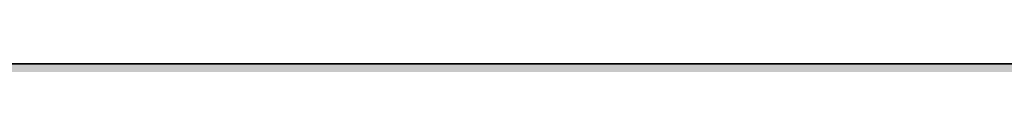
# Model space of a CAD drawing. Units: inches. Extents: x 2091 to 2899, y 967 to 2217.
# Tile 81 of 256: x 2238.361 to 2245.941, y 1099.919 to 1099.919. Entities that reach past the tile are written whole.
import ezdxf

# ---------------------------------------------------------------- set-up
doc = ezdxf.new("R2010")
doc.units = ezdxf.units.IN
doc.layers.add('A-WALL-PATT', color=141, linetype='Continuous', lineweight=13, true_color=0xadddf7)
doc.layers.add('L-SITE-WALL', color=7, linetype='Continuous', lineweight=35)

msp = doc.modelspace()

# ---------------------------------------------------------------- hatches: boundary and pattern name
at = {"layer": 'A-WALL-PATT'}
h = msp.add_hatch(color=256, dxfattribs=at)
h.dxf.hatch_style = 1
h.paths.add_polyline_path([(2212.1436, 1941.4191), (2387.6436, 1941.4191), (2387.6436, 1824.4191), (2392.1436, 1824.4191), (2392.1436, 1941.4191), (2609.6436, 1941.4191), (2609.6436, 1825.9191), (2614.1436, 1825.9191), (2614.1436, 1941.4191), (2794.1436, 1941.4191), (2794.1436, 1928.7622), (2803.1436, 1928.7622), (2803.1436, 2050.9191), (2203.1436, 2050.9191), (2203.1436, 1900.7579), (2212.1436, 1900.7579)])
h.paths.add_polyline_path([(2212.1436, 1945.9191), (2212.1436, 2041.9191), (2794.1436, 2041.9191), (2794.1436, 1945.9191), (2402.2482, 1945.9191), (2401.1024, 1945.7758), (2398.7024, 1945.7758)], flags=16)
h.paths.add_polyline_path([(2230.2299, 1948.0628), (2227.3499, 1949.5028), (2225.9099, 1951.9028), (2223.9899, 1952.8628), (2223.0299, 1955.2628), (2222.0699, 1959.5828), (2222.0699, 1963.4228), (2223.0299, 1965.6628), (2223.9899, 1965.3428), (2225.5859, 1963.8607), (2226.9115, 1964.9573), (2226.9489, 1965.9388), (2227.7783, 1966.9521), (2228.1999, 1968.8787), (2230.7099, 1964.8628), (2233.5899, 1966.3028), (2233.6073, 1966.3319), (2233.7727, 1964.9382), (2234.6338, 1963.6765), (2235.0299, 1963.9028), (2236.282, 1965.5724), (2235.9899, 1962.9428), (2237.9545, 1957.54), (2238.3899, 1957.9028), (2239.2159, 1960.3058), (2238.6546, 1966.385), (2238.6928, 1966.4381), (2238.8406, 1967.4997), (2238.7803, 1967.6875), (2238.8805, 1967.7868), (2238.6669, 1966.2518), (2239.2159, 1960.3058), (2238.3899, 1957.9028), (2236.9499, 1956.7028), (2234.5499, 1949.9828)], flags=0)
h.paths.add_polyline_path([(2278.012, 1948.0628), (2276.4964, 1947.8733), (2275.8498, 1947.6886), (2274.652, 1947.1028)], flags=0)
h.paths.add_polyline_path([(2269.852, 1955.7428), (2268.2762, 1956.6293), (2270.8673, 1956.3484), (2269.372, 1958.1428), (2268.715, 1959.1923), (2270.5698, 1958.7286), (2268.5807, 1961.9061), (2270.812, 1960.8919), (2270.812, 1963.4228), (2271.3933, 1964.7793), (2270.2918, 1966.1562), (2271.772, 1965.6628), (2272.1414, 1966.5248), (2273.9298, 1965.9286), (2275.6304, 1968.0543), (2276.3319, 1966.7219), (2276.5204, 1966.9521), (2276.942, 1968.8787), (2277.7343, 1967.6111), (2278.1399, 1969.4645), (2279.6591, 1967.0337), (2280.412, 1966.7828), (2280.9493, 1967.5888), (2281.6098, 1967.3686), (2282.1333, 1968.1538), (2282.3492, 1966.3334), (2282.3498, 1966.3326), (2283.4076, 1968.0954), (2283.7126, 1965.524), (2284.3202, 1964.6338), (2284.5118, 1964.8892), (2284.235, 1965.7048), (2284.5005, 1967.319), (2284.9079, 1965.4174), (2285.3963, 1966.0686), (2285.4328, 1966.2906), (2285.4733, 1966.1713), (2286.3539, 1967.3454), (2286.222, 1966.1582), (2287.6635, 1968.0802), (2287.714, 1968.4428), (2288.4816, 1969.0167), (2288.574, 1968.7289), (2288.9175, 1969.069), (2288.6068, 1966.8376), (2288.9287, 1963.3513), (2288.935, 1963.3568), (2288.9297, 1963.3404), (2289.0153, 1962.4139), (2290.1112, 1963.8751), (2290.1328, 1963.9426), (2290.2177, 1964.0171), (2290.1112, 1963.8751), (2289.1558, 1960.8916), (2288.594, 1959.2572), (2288.572, 1959.1028), (2289.532, 1960.5428), (2290.012, 1962.4628), (2290.1918, 1962.6427), (2289.7698, 1959.6886), (2286.8898, 1957.2886), (2284.4898, 1950.5686), (2283.3147, 1950.0463), (2283.292, 1949.9828), (2280.2901, 1948.6486), (2281.1298, 1948.6486), (2282.5698, 1948.1686), (2283.2047, 1948.0628), (2278.972, 1948.0628), (2276.092, 1949.5028), (2274.652, 1951.9028), (2272.732, 1952.8628)], flags=0)
h.paths.add_polyline_path([(2271.1589, 1958.0218), (2272.9698, 1955.8486), (2272.0098, 1960.1686), (2272.0098, 1964.0086), (2272.6244, 1965.4427), (2274.328, 1963.8607), (2275.6536, 1964.9573), (2275.6377, 1964.5391), (2277.4122, 1966.0069), (2277.033, 1965.1568), (2276.8299, 1964.9756), (2276.766, 1963.295), (2277.4496, 1962.6602), (2279.452, 1964.8628), (2282.332, 1966.3028), (2283.5298, 1966.8886), (2283.2945, 1966.7709), (2283.913, 1963.8847), (2284.8992, 1964.4483), (2284.732, 1962.9428), (2286.6966, 1957.54), (2287.132, 1957.9028), (2287.5419, 1959.0954), (2287.7794, 1958.4423), (2285.6827, 1956.6951), (2285.8765, 1959.7953), (2284.732, 1962.9428), (2284.8992, 1964.4483), (2283.913, 1963.8847), (2284.2238, 1962.4341), (2283.4244, 1963.6055), (2281.6098, 1962.5686), (2281.1298, 1960.1686), (2282.0898, 1956.3286), (2283.0498, 1952.9686), (2282.5698, 1950.5686), (2280.1698, 1948.6486), (2279.8833, 1948.7919), (2278.972, 1948.0628), (2278.972, 1949.0228), (2278.6723, 1949.3974), (2277.2898, 1950.0886), (2275.8498, 1952.4886), (2273.9298, 1953.4486), (2272.4898, 1954.8886), (2271.9216, 1954.8886), (2271.772, 1955.2628)], flags=0)
h.paths.add_polyline_path([(2311.9941, 1955.7428), (2312.0627, 1955.6742), (2312.0551, 1955.7085)], flags=0)
h.paths.add_polyline_path([(2331.9561, 1963.9518), (2333.3961, 1965.3918), (2331.0771, 1963.3568), (2330.9986, 1963.1115)], flags=0)
h.paths.add_polyline_path([(2310.5541, 1954.3028), (2307.0398, 1956.2799), (2310.7629, 1955.8763), (2312.4741, 1953.8228), (2313.4341, 1951.4228), (2315.3541, 1950.4628), (2316.7941, 1948.0628), (2317.4661, 1947.7268), (2319.3687, 1947.9646), (2317.7541, 1949.9828), (2317.5695, 1950.6105), (2316.7941, 1951.9028), (2314.8741, 1952.8628), (2313.9141, 1955.2628), (2311.5141, 1958.1428), (2309.3755, 1961.5592), (2311.5141, 1960.3371), (2311.5141, 1961.9828), (2310.6047, 1963.1196), (2311.7266, 1962.4785), (2312.4183, 1964.0926), (2312.256, 1964.2955), (2313.1941, 1963.9828), (2313.9141, 1965.6628), (2314.6468, 1965.4186), (2315.3541, 1966.3028), (2316.7941, 1967.7428), (2316.1574, 1966.9469), (2317.0341, 1965.2819), (2317.2226, 1965.5121), (2317.777, 1968.0458), (2318.4741, 1966.7219), (2318.6626, 1966.9521), (2319.0842, 1968.8787), (2321.207, 1965.4821), (2322.1614, 1966.9137), (2322.5541, 1966.7828), (2322.786, 1967.1306), (2322.8816, 1966.3243), (2323.312, 1965.7217), (2323.6513, 1965.8914), (2324.3965, 1967.1334), (2324.6569, 1964.9382), (2324.972, 1964.4766), (2325.3873, 1967.0015), (2325.9408, 1964.4183), (2327.2289, 1966.1358), (2327.1663, 1965.5724), (2328.0591, 1966.7628), (2328.2246, 1966.2475), (2329.668, 1967.6769), (2329.6646, 1967.6875), (2329.7648, 1967.7868), (2329.5511, 1966.2518), (2330.1001, 1960.3058), (2329.3328, 1958.0735), (2329.3131, 1957.9352), (2329.6341, 1958.2028), (2330.2341, 1959.1028), (2330.7141, 1961.0228), (2331.0341, 1961.3428), (2330.7141, 1959.1028), (2329.6341, 1958.2028), (2329.2741, 1957.6628), (2327.7121, 1956.3611), (2325.4341, 1949.9828), (2324.3338, 1949.4937), (2323.9941, 1948.5428), (2319.6741, 1946.6228), (2316.7941, 1948.0628), (2315.3541, 1950.4628), (2313.4341, 1951.4228)], flags=0)
h.paths.add_polyline_path([(2321.3357, 1947.952), (2321.1141, 1948.0628), (2321.1141, 1949.0228), (2319.1941, 1951.4228), (2316.7941, 1959.5828), (2316.6632, 1959.5828), (2315.3541, 1958.1428), (2314.3941, 1958.1428), (2313.1483, 1958.7091), (2312.9541, 1959.5828), (2312.9541, 1960.8919), (2315.8341, 1959.5828), (2316.6632, 1959.5828), (2317.3147, 1960.2994), (2315.0302, 1962.4207), (2316.3558, 1963.5173), (2316.3723, 1963.9516), (2316.4702, 1963.8607), (2317.7958, 1964.9573), (2317.7552, 1963.8897), (2319.1751, 1965.1568), (2319.4984, 1965.8814), (2321.1141, 1965.3428), (2323.2359, 1962.3724), (2325.6863, 1963.7726), (2325.5428, 1962.4806), (2325.1988, 1963.494), (2324.4785, 1963.0824), (2324.926, 1960.9941), (2324.0781, 1962.2365), (2322.4148, 1961.286), (2322.0741, 1959.5828), (2323.0341, 1955.7428), (2323.9941, 1952.3828), (2323.5141, 1949.9828), (2322.1427, 1948.8856), (2322.0741, 1948.5428)], flags=0)
h.paths.add_polyline_path([(2320.2075, 1963.3375), (2320.1541, 1963.4228), (2320.3941, 1963.5428)], flags=0)
h.paths.add_polyline_path([(2353.8505, 1965.8105), (2354.0305, 1965.7505), (2354.3305, 1966.4505), (2354.3305, 1966.9305)], flags=0)
h.paths.add_polyline_path([(2359.0206, 1969.0264), (2359.0984, 1968.9019), (2359.2335, 1969.5195), (2359.2335, 1969.9995)], flags=0)
h.paths.add_polyline_path([(2358.2567, 1966.6817), (2357.9836, 1966.348), (2358.2113, 1966.1462), (2358.4105, 1966.3896)], flags=0)
h.paths.add_polyline_path([(2357.7685, 1966.0588), (2357.7322, 1965.105), (2357.751, 1965.1206), (2357.7695, 1965.6065), (2357.7695, 1966.0578)], flags=0)
h.paths.add_polyline_path([(2359.1115, 1965.3045), (2359.1115, 1964.8245), (2359.8445, 1966.4675), (2359.8445, 1966.9475)], flags=0)
h.paths.add_polyline_path([(2360.2237, 1966.6214), (2360.6985, 1969.3625), (2360.6985, 1969.8425), (2360.2105, 1967.0255), (2360.2105, 1966.6425)], flags=0)
h.paths.add_polyline_path([(2363.4505, 1967.8905), (2363.4505, 1968.3705), (2362.4905, 1966.9305), (2362.656, 1966.6988)], flags=0)
h.paths.add_polyline_path([(2364.4755, 1966.0788), (2365.8505, 1968.3705), (2365.8505, 1968.8505), (2364.428, 1966.4796)], flags=0)
h.paths.add_polyline_path([(2366.3135, 1965.8525), (2366.3667, 1965.6958), (2366.8025, 1968.3455), (2366.8025, 1968.8255)], flags=0)
h.paths.add_polyline_path([(2367.1653, 1965.8035), (2367.2905, 1966.9305), (2367.2905, 1967.4105), (2367.1027, 1965.7201)], flags=0)
h.paths.add_polyline_path([(2370.0365, 1959.9735), (2371.0135, 1963.0245), (2371.0135, 1963.5045), (2370.0365, 1960.4535)], flags=0)
h.paths.add_polyline_path([(2371.6105, 1960.2105), (2372.5705, 1961.6505), (2372.5705, 1962.1305), (2371.8025, 1960.9785)], flags=0)
h.paths.add_polyline_path([(2350.8737, 1956.0051), (2351.9305, 1955.8905), (2354.4905, 1953.3305), (2353.8505, 1954.9305), (2351.4505, 1957.8105), (2347.9355, 1963.4255), (2347.9355, 1963.9055), (2351.4505, 1958.2905), (2353.7051, 1955.585), (2352.8905, 1959.2505), (2352.8905, 1959.7305), (2352.8905, 1961.9248), (2356.7305, 1959.7305), (2358.4545, 1961.6268), (2354.8105, 1965.0105), (2355.0309, 1965.2859), (2358.6911, 1961.8871), (2361.5305, 1965.0105), (2364.3765, 1966.4335), (2364.5244, 1965.1869), (2365.4545, 1963.8242), (2365.8811, 1964.068), (2365.3705, 1966.4505), (2365.3705, 1966.9305), (2366.8105, 1960.2105), (2366.8105, 1959.7305), (2366.3887, 1952.9814), (2367.7705, 1956.8505), (2368.6412, 1957.5761), (2366.8105, 1962.6105), (2366.8105, 1963.0905), (2368.7752, 1957.6877), (2369.2105, 1958.0505), (2370.0016, 1960.3519), (2369.4752, 1966.0527), (2369.5135, 1966.1058), (2369.5142, 1966.1109), (2369.4752, 1966.5327), (2369.5135, 1966.5858), (2369.6146, 1967.3126), (2369.1825, 1968.6585), (2369.1825, 1969.1385), (2369.601, 1967.8352), (2369.7012, 1967.9345), (2369.7179, 1968.0547), (2370.1452, 1968.3741), (2369.7787, 1968.0112), (2369.7012, 1967.4545), (2370.4682, 1968.214), (2369.6749, 1967.2658), (2369.5142, 1966.1109), (2370.0365, 1960.4535), (2370.0365, 1959.9735), (2369.4418, 1958.2432), (2370.6505, 1959.2505), (2371.0458, 1962.0176), (2371.1305, 1962.1305), (2370.6505, 1958.7705), (2367.7705, 1956.3705), (2365.3705, 1949.6505), (2362.0791, 1948.1876), (2363.4505, 1947.7305), (2361.0505, 1947.7305), (2360.0905, 1947.7305), (2357.1039, 1947.3572), (2360.0905, 1948.2105), (2358.1705, 1949.1705), (2356.7305, 1951.5705), (2354.8105, 1952.5305), (2351.9305, 1955.4105)], flags=0)
h.paths.add_polyline_path([(2361.0505, 1948.6905), (2359.1305, 1951.0905), (2356.7305, 1959.2505), (2355.7705, 1959.2505), (2352.8905, 1960.5596), (2352.8905, 1961.4448), (2355.8905, 1959.7305), (2356.7305, 1959.7305), (2356.8372, 1959.3678), (2361.5305, 1964.5305), (2363.2484, 1965.3894), (2364.9253, 1963.0418), (2362.4905, 1961.6505), (2362.0639, 1959.5172), (2362.9705, 1955.8905), (2363.9305, 1952.5305), (2363.9305, 1952.0505), (2363.4505, 1949.6505), (2361.0505, 1947.7305)], flags=0)
h.paths.add_polyline_path([(2359.1305, 1951.5705), (2359.2905, 1951.3705), (2361.0505, 1954.4505), (2361.0505, 1954.9305)], flags=0)
h.paths.add_polyline_path([(2357.2195, 1966.5455), (2356.7925, 1968.8145), (2356.7925, 1969.2945), (2357.2195, 1967.0255)], flags=0)
h.paths.add_polyline_path([(2361.0505, 1954.4505), (2361.5305, 1958.7705), (2361.5305, 1959.2505), (2361.0505, 1954.9305)], flags=0)
h.paths.add_polyline_path([(2402.5483, 1948.4861), (2402.3024, 1948.4158), (2402.5904, 1948.4158)], flags=0)
h.paths.add_polyline_path([(2394.1424, 1956.0958), (2395.6851, 1954.5532), (2396.7205, 1953.9707), (2396.0624, 1955.6158), (2395.2414, 1956.6011), (2395.8789, 1956.4417), (2395.1024, 1959.9358), (2395.1024, 1963.7758), (2396.0624, 1966.0158), (2397.0224, 1965.6958), (2398.6185, 1964.2138), (2399.9441, 1965.3103), (2399.9814, 1966.2918), (2400.8109, 1967.3052), (2401.2325, 1969.2317), (2403.5379, 1965.543), (2403.942, 1967.3893), (2404.7024, 1967.1358), (2405.4603, 1966.0748), (2406.6224, 1966.6558), (2406.6399, 1966.6849), (2406.8052, 1965.2912), (2406.9257, 1965.1147), (2407.3424, 1964.9758), (2407.8743, 1965.7737), (2408.1691, 1964.3981), (2409.3146, 1965.9254), (2409.2175, 1965.0511), (2409.4452, 1963.1312), (2410.3064, 1961.8695), (2410.7024, 1962.0958), (2411.4423, 1963.0823), (2411.1654, 1963.8978), (2411.6164, 1966.6398), (2411.7254, 1966.7911), (2411.8732, 1967.8527), (2411.8129, 1968.0405), (2411.9131, 1968.1398), (2411.6994, 1966.6048), (2412.2484, 1960.6588), (2413.2254, 1963.7098), (2414.3779, 1964.7212), (2414.5132, 1965.6927), (2414.4529, 1965.8805), (2414.5531, 1965.9798), (2414.3779, 1964.7212), (2414.5198, 1964.8457), (2414.3654, 1964.6311), (2414.3394, 1964.4448), (2414.8884, 1958.4988), (2414.0624, 1956.0958), (2412.6224, 1954.8958), (2410.1714, 1948.0329), (2410.0167, 1948.0844), (2405.9024, 1946.2558), (2405.9024, 1947.2158), (2405.2043, 1948.0886), (2404.2224, 1948.4158), (2403.2624, 1948.4158), (2400.3824, 1949.8558), (2399.6624, 1951.0558), (2397.9824, 1952.7358), (2397.0224, 1953.2158), (2395.6851, 1954.5532), (2392.6568, 1956.2569)], flags=0)
h.paths.add_polyline_path([(2409.0857, 1964.4074), (2409.1304, 1964.2757), (2409.2624, 1964.4958)], flags=0)
h.paths.add_polyline_path([(2397.7424, 1961.6158), (2398.7024, 1963.8558), (2399.6624, 1963.5358), (2401.4266, 1965.741), (2401.7914, 1966.5588), (2402.0714, 1965.0708), (2402.8355, 1964.3934), (2403.2624, 1964.9149), (2403.3381, 1964.7711), (2402.6155, 1963.9762), (2402.4986, 1960.9022), (2403.543, 1959.9325), (2404.4132, 1960.8897), (2404.7024, 1962.3358), (2407.9163, 1964.1724), (2409.5202, 1961.9269), (2410.9871, 1957.893), (2411.4224, 1958.2558), (2412.048, 1960.0756), (2412.4103, 1959.0791), (2411.6756, 1958.4668), (2411.6624, 1958.2558), (2411.6261, 1958.4255), (2409.9824, 1957.0558), (2407.5824, 1950.3358), (2403.2624, 1948.4158), (2403.2624, 1949.3758), (2401.3424, 1951.7758), (2399.4165, 1958.324), (2397.7424, 1959.0849), (2397.7424, 1959.9701), (2397.1024, 1960.3358), (2397.7424, 1960.0449)], flags=0)
h.paths.add_polyline_path([(2405.9024, 1952.9758), (2405.9504, 1953.4078), (2406.0167, 1953.1758)], flags=0)
h.paths.add_polyline_path([(2449.8178, 1967.114), (2449.7523, 1967.1358), (2449.7937, 1967.0779)], flags=0)
h.paths.add_polyline_path([(2451.6977, 1966.6181), (2451.7409, 1966.6901), (2451.6921, 1966.6657)], flags=0)
h.paths.add_polyline_path([(2454.3436, 1965.7376), (2455.7523, 1967.6158), (2455.9923, 1968.0958), (2454.3645, 1965.9254)], flags=0)
h.paths.add_polyline_path([(2457.5473, 1968.8638), (2457.7873, 1969.3438), (2457.0543, 1968.7958), (2457.0076, 1968.4603)], flags=0)
h.paths.add_polyline_path([(2456.9218, 1967.8567), (2456.8022, 1968.229), (2456.723, 1967.6598)], flags=0)
h.paths.add_polyline_path([(2457.3023, 1967.3768), (2457.5423, 1967.8568), (2456.8103, 1966.8398), (2456.7405, 1966.7002), (2456.749, 1966.6081)], flags=0)
h.paths.add_polyline_path([(2458.2753, 1963.7098), (2458.1553, 1963.3352), (2460.3543, 1965.2648), (2460.5943, 1965.7448)], flags=0)
h.paths.add_polyline_path([(2458.3923, 1962.8158), (2458.3641, 1962.6182), (2459.5923, 1964.2558), (2459.8323, 1964.7358)], flags=0)
h.paths.add_polyline_path([(2459.3523, 1962.8158), (2459.2723, 1962.4958), (2460.0723, 1963.2958), (2460.3123, 1963.7758)], flags=0)
h.paths.add_polyline_path([(2458.6803, 1960.6078), (2458.6323, 1960.4158), (2459.5923, 1961.8558), (2459.8323, 1962.3358)], flags=0)
h.paths.add_polyline_path([(2437.8382, 1956.2427), (2439.1923, 1956.0958), (2441.3523, 1953.9358), (2440.8723, 1955.1358), (2438.4723, 1958.0158), (2438.0716, 1958.656), (2438.7123, 1958.4958), (2440.6396, 1956.1831), (2439.9123, 1959.4558), (2439.9123, 1963.2958), (2441.3523, 1966.6558), (2441.5923, 1967.1358), (2441.1123, 1966.0158), (2442.0723, 1965.6958), (2443.989, 1968.0917), (2444.2413, 1966.7508), (2444.9168, 1966.1519), (2445.6766, 1967.0801), (2446.2553, 1969.7248), (2446.4953, 1970.2048), (2446.2824, 1969.2317), (2447.3627, 1967.5033), (2447.7203, 1969.5678), (2447.9603, 1970.0478), (2447.4855, 1967.3068), (2448.7923, 1965.2158), (2448.4723, 1964.8638), (2448.5523, 1964.7358), (2451.4521, 1966.1857), (2451.6151, 1964.8112), (2452.3079, 1963.7962), (2453.2345, 1964.3257), (2454.0723, 1960.4158), (2453.6287, 1953.3177), (2454.7923, 1956.5758), (2455.0323, 1957.0558), (2455.7188, 1957.6279), (2453.8323, 1962.8158), (2453.941, 1963.7936), (2453.3353, 1965.5778), (2453.8243, 1968.5508), (2454.0643, 1969.0308), (2453.5753, 1966.0578), (2454.0403, 1964.6879), (2453.8323, 1962.8158), (2455.7188, 1957.6279), (2456.3672, 1958.1682), (2457.0583, 1960.1788), (2457.2983, 1960.6588), (2456.4723, 1958.2558), (2457.7177, 1959.2937), (2457.6723, 1958.9758), (2454.89, 1956.6572), (2453.6141, 1953.0849), (2453.5923, 1952.7358), (2453.3523, 1952.2558), (2453.3596, 1952.3722), (2452.6323, 1950.3358), (2452.3923, 1949.8558), (2449.2038, 1948.4387), (2450.7123, 1947.9358), (2448.0723, 1947.9358), (2447.1123, 1947.9358), (2444.5523, 1947.6158), (2447.1996, 1948.3722), (2445.1923, 1949.3758), (2443.7523, 1951.7758), (2441.8323, 1952.7358), (2438.9523, 1955.6158)], flags=0)
h.paths.add_polyline_path([(2443.9923, 1959.9358), (2444.0403, 1959.7726), (2444.1216, 1959.862)], flags=0)
h.paths.add_polyline_path([(2442.9123, 1959.9358), (2443.0323, 1959.9358), (2442.4457, 1960.2025)], flags=0)
h.paths.add_polyline_path([(2444.9829, 1965.0197), (2445.2793, 1965.2648), (2445.5193, 1965.7448), (2444.994, 1965.3103)], flags=0)
h.paths.add_polyline_path([(2446.1333, 1965.0298), (2446.3304, 1965.4715), (2444.9703, 1964.2578), (2444.7303, 1963.7778)], flags=0)
h.paths.add_polyline_path([(2442.7923, 1959.4558), (2443.7523, 1959.4558), (2446.1523, 1951.2958), (2446.4123, 1951.7508), (2446.3923, 1951.7758), (2448.0806, 1954.7303), (2448.5523, 1958.9758), (2441.8323, 1965.2158), (2442.1549, 1965.6191), (2448.7923, 1959.4558), (2448.3123, 1955.1358), (2448.0723, 1954.6558), (2446.4123, 1951.7508), (2448.3123, 1949.3758), (2448.3123, 1948.4158), (2450.5409, 1950.1987), (2450.9523, 1952.2558), (2449.9923, 1955.6158), (2449.0323, 1959.4558), (2449.5123, 1961.8558), (2449.7523, 1962.3358), (2449.6749, 1961.9487), (2452.9945, 1963.8457), (2453.0644, 1963.5194), (2452.8846, 1963.7829), (2449.6749, 1961.9487), (2449.2723, 1959.9358), (2450.2323, 1956.0958), (2451.1923, 1952.7358), (2450.7123, 1950.3358), (2450.4723, 1949.8558), (2448.0723, 1947.9358), (2448.0723, 1948.5358), (2445.4323, 1949.8558), (2443.9923, 1952.2558), (2442.0723, 1953.2158), (2441.1123, 1955.6158), (2440.1523, 1959.9358), (2440.1523, 1960.6558)], flags=0)
h.paths.add_polyline_path([(2456.6923, 1966.9858), (2457.6083, 1968.0808), (2457.8483, 1968.5608), (2456.9323, 1967.4658)], flags=0)
h.paths.add_polyline_path([(2489.8966, 1966.5802), (2489.9429, 1966.1893), (2490.7475, 1967.5302), (2491.3191, 1968.9512)], flags=0)
h.paths.add_polyline_path([(2473.5625, 1956.4071), (2477.14, 1956.0193), (2476.9553, 1956.2408), (2475.108, 1957.2801), (2476.3475, 1956.9702), (2475.1869, 1958.8242), (2476.9191, 1958.3912), (2475.4116, 1960.7993), (2477.7875, 1959.7193), (2477.7875, 1962.2502), (2477.6374, 1962.4379), (2477.8226, 1962.3321), (2478.3591, 1963.5841), (2478.3591, 1963.6712), (2477.3243, 1964.9646), (2478.7148, 1964.5011), (2479.3191, 1965.9112), (2480.2791, 1965.5912), (2481.784, 1967.4722), (2482.1165, 1965.7052), (2482.8806, 1965.0278), (2483.2093, 1965.4294), (2483.2202, 1965.7151), (2483.0759, 1965.989), (2483.7118, 1966.7658), (2484.1305, 1968.6792), (2484.7021, 1970.1002), (2484.4892, 1969.1271), (2486.5029, 1965.9051), (2487.3875, 1965.6102), (2488.1534, 1966.7591), (2488.717, 1965.9701), (2489.2001, 1966.2116), (2489.3307, 1965.111), (2490.3939, 1963.6225), (2490.6608, 1963.775), (2490.4939, 1964.5536), (2490.9231, 1963.9248), (2491.3191, 1964.1512), (2491.3334, 1964.1702), (2491.2105, 1964.5322), (2491.2818, 1964.9655), (2491.4258, 1964.2934), (2494.0765, 1967.8276), (2494.4979, 1966.5149), (2494.5982, 1966.6142), (2494.6895, 1967.2702), (2495.1067, 1967.5822), (2495.1298, 1967.7481), (2495.0696, 1967.9359), (2495.1698, 1968.0351), (2495.0318, 1967.0436), (2495.7538, 1967.7587), (2494.9821, 1966.6864), (2494.9561, 1966.5002), (2495.479, 1960.8369), (2495.9105, 1962.1842), (2496.4821, 1963.6052), (2496.0727, 1962.3266), (2496.7689, 1962.9375), (2496.5991, 1962.7112), (2496.1191, 1959.3512), (2496.7329, 1960.2718), (2496.9875, 1961.2902), (2497.5591, 1962.7112), (2497.0791, 1960.7912), (2496.5075, 1959.3702), (2495.5475, 1957.9302), (2492.7588, 1955.6064), (2490.8391, 1950.2312), (2490.2675, 1948.8102), (2485.9475, 1946.8902), (2483.0675, 1948.3302), (2481.6275, 1950.7302), (2479.7075, 1951.6902), (2476.8275, 1954.5702)], flags=0)
h.paths.add_polyline_path([(2485.577, 1948.3134), (2485.5591, 1948.3112), (2485.5788, 1948.3112)], flags=0)
h.paths.add_polyline_path([(2478.6451, 1954.5512), (2478.109, 1956.9633), (2479.3191, 1955.5112), (2480.2791, 1953.1112), (2482.1991, 1952.1512), (2483.6391, 1949.7512), (2486.5191, 1948.3112), (2486.5191, 1949.2712), (2484.7393, 1951.4959), (2484.0275, 1950.2502), (2481.6275, 1958.4102), (2482.3751, 1959.2327), (2482.1991, 1959.8312), (2483.1976, 1960.9295), (2479.7075, 1964.1702), (2480.6034, 1965.2901), (2481.8752, 1964.1091), (2482.6664, 1964.7636), (2482.6154, 1963.4218), (2482.9892, 1963.0747), (2484.0085, 1963.9842), (2484.6836, 1965.4975), (2484.5801, 1965.4052), (2485.3573, 1967.1471), (2485.1206, 1965.7812), (2486.4275, 1963.6902), (2488.1454, 1964.5492), (2489.8223, 1962.2016), (2490.7475, 1962.7302), (2491.9997, 1964.3998), (2492.076, 1965.0873), (2492.2129, 1964.6841), (2492.4854, 1965.0474), (2492.2791, 1963.1912), (2494.2438, 1957.7884), (2494.5625, 1958.054), (2494.9335, 1959.1332), (2495.5051, 1960.5542), (2494.6791, 1958.1512), (2494.1075, 1956.7302), (2494.5625, 1958.054), (2493.4085, 1957.0923), (2491.7075, 1961.7702), (2491.9997, 1964.3998), (2490.7475, 1962.7302), (2487.712, 1960.9957), (2487.4791, 1959.8312), (2488.4391, 1955.9912), (2489.3991, 1952.6312), (2488.9191, 1950.2312), (2488.5769, 1949.9574), (2488.3475, 1948.8102), (2487.6517, 1948.2536), (2487.4791, 1948.3112), (2486.5191, 1948.3112), (2483.6391, 1949.7512), (2482.1991, 1952.1512), (2480.2791, 1953.1112), (2478.8391, 1954.5512)], flags=0)
h.paths.add_polyline_path([(2526.6483, 1966.9875), (2526.5173, 1967.0312), (2526.6001, 1966.9153)], flags=0)
h.paths.add_polyline_path([(2528.4706, 1966.4467), (2528.5745, 1966.6197), (2528.4571, 1966.561)], flags=0)
h.paths.add_polyline_path([(2534.1333, 1967.4962), (2534.1567, 1967.5428), (2534.0598, 1967.4083)], flags=0)
h.paths.add_polyline_path([(2536.1619, 1964.0506), (2535.1573, 1962.7112), (2535.1009, 1962.3159), (2536.1173, 1963.6712), (2536.4205, 1964.2775)], flags=0)
h.paths.add_polyline_path([(2535.1573, 1959.8312), (2536.1173, 1961.2712), (2536.5973, 1962.2312), (2535.2533, 1960.2152)], flags=0)
h.paths.add_polyline_path([(2513.249, 1956.2848), (2516.2212, 1955.9626), (2514.9973, 1957.4312), (2514.1958, 1958.7115), (2515.4773, 1958.3912), (2516.9319, 1956.6457), (2516.4373, 1958.8712), (2516.4373, 1962.7112), (2516.8727, 1963.727), (2515.3464, 1965.6348), (2517.3973, 1964.9512), (2517.8773, 1966.0712), (2518.3573, 1967.0312), (2517.8773, 1965.9112), (2518.8373, 1965.5912), (2520.4866, 1967.6527), (2520.7663, 1966.1662), (2521.5304, 1965.4887), (2521.7814, 1965.7954), (2521.8009, 1966.3073), (2521.4778, 1966.9209), (2521.2463, 1967.1262), (2521.1777, 1967.4909), (2521.4778, 1966.9209), (2522.0104, 1966.4487), (2522.2574, 1966.7504), (2522.7803, 1969.1402), (2523.2603, 1970.1002), (2523.0474, 1969.1271), (2524.6731, 1966.5259), (2526.0373, 1966.0712), (2526.7952, 1965.0101), (2527.9771, 1965.601), (2528.1401, 1964.2266), (2528.6646, 1963.4582), (2529.3886, 1963.8719), (2529.3297, 1964.147), (2529.4813, 1963.9248), (2529.8773, 1964.1512), (2529.984, 1964.2934), (2529.7891, 1965.2032), (2530.0624, 1964.3979), (2532.8025, 1968.0513), (2533.1478, 1966.9759), (2533.248, 1967.0751), (2533.3393, 1967.7312), (2533.6728, 1967.9805), (2533.728, 1968.0351), (2533.5143, 1966.5002), (2534.0247, 1960.9725), (2534.5603, 1962.6452), (2535.0403, 1963.6052), (2534.0633, 1960.5542), (2533.2373, 1958.1512), (2534.2882, 1959.0268), (2534.1973, 1958.3912), (2531.5126, 1956.1539), (2529.3973, 1950.2312), (2528.9173, 1949.2712), (2526.4488, 1948.174), (2527.4773, 1947.8312), (2530.3573, 1947.3512), (2524.5973, 1947.3512), (2521.7173, 1948.7912), (2520.2773, 1951.1912), (2518.3573, 1952.1512), (2515.4773, 1955.0312)], flags=0)
h.paths.add_polyline_path([(2523.9348, 1967.1903), (2523.6195, 1966.4837), (2523.7705, 1966.2421)], flags=0)
h.paths.add_polyline_path([(2518.8373, 1953.1112), (2517.8773, 1955.5112), (2516.885, 1959.9768), (2516.9173, 1959.9621), (2516.9173, 1962.0254), (2520.7573, 1959.8312), (2522.0249, 1961.2255), (2518.3573, 1964.6312), (2519.0026, 1965.4377), (2520.4334, 1964.1091), (2521.3011, 1964.8269), (2521.2452, 1963.3553), (2525.6383, 1959.276), (2526.0373, 1961.2712), (2529.3973, 1963.1912), (2530.6495, 1964.8607), (2530.6647, 1964.9976), (2530.692, 1964.9173), (2531.0878, 1965.4451), (2530.946, 1964.1689), (2530.692, 1964.9173), (2529.3973, 1963.1912), (2526.3625, 1961.457), (2526.0373, 1959.8312), (2526.9973, 1955.9912), (2527.9573, 1952.6312), (2527.4773, 1950.2312), (2527.1345, 1949.9569), (2526.9739, 1949.1541), (2526.6973, 1949.0312), (2524.5973, 1947.3512), (2524.5973, 1948.3112), (2524.2773, 1948.7112), (2522.1973, 1949.7512), (2520.7573, 1952.1512)], flags=0)
h.paths.add_polyline_path([(2520.2773, 1958.8712), (2520.8533, 1959.5048), (2523.1573, 1951.6712), (2524.6139, 1954.2201), (2524.5973, 1954.0712), (2522.6773, 1950.7112)], flags=0)
h.paths.add_polyline_path([(2559.3709, 1966.3112), (2559.3984, 1966.3249), (2559.4019, 1966.3453)], flags=0)
h.paths.add_polyline_path([(2549.7709, 1957.1912), (2552.6509, 1954.3112), (2552.134, 1955.6035), (2550.6109, 1957.4312), (2547.0959, 1963.0462), (2545.7759, 1965.2062), (2549.2909, 1959.5912), (2551.6909, 1956.7112), (2550.7929, 1960.7521), (2550.7309, 1960.7803), (2550.7309, 1964.8712), (2551.6909, 1967.1112), (2552.6509, 1966.7912), (2554.247, 1965.3091), (2555.0343, 1965.9603), (2555.5817, 1966.6446), (2555.6099, 1967.3872), (2556.4394, 1968.4005), (2556.861, 1970.3271), (2559.3709, 1966.3112), (2560.6909, 1964.1512), (2562.4088, 1965.0101), (2561.6509, 1966.0712), (2560.3309, 1968.2312), (2561.7585, 1966.2325), (2562.3472, 1967.1156), (2562.4337, 1966.3866), (2563.1278, 1965.3696), (2563.5709, 1965.5912), (2563.5884, 1965.6202), (2563.3625, 1967.5235), (2563.7225, 1965.8438), (2565.06, 1968.073), (2564.7329, 1965.1287), (2565.1176, 1963.3334), (2567.4446, 1966.4361), (2567.3156, 1967.8333), (2567.3538, 1967.8864), (2567.5016, 1968.9481), (2567.4413, 1969.1359), (2567.5416, 1969.2351), (2567.3279, 1967.7002), (2567.8769, 1961.7542), (2568.7467, 1964.4703), (2568.6356, 1965.6733), (2568.6738, 1965.7264), (2568.8216, 1966.7881), (2568.7613, 1966.9759), (2568.8616, 1967.0751), (2568.6479, 1965.5402), (2568.7261, 1964.693), (2568.8539, 1964.8052), (2568.7467, 1964.4703), (2568.8172, 1963.7063), (2568.9709, 1963.9112), (2568.8661, 1963.1773), (2569.1969, 1959.5942), (2568.3709, 1957.1912), (2566.9309, 1955.9912), (2564.6203, 1949.5214), (2564.6509, 1949.5112), (2564.6166, 1949.5112), (2564.5309, 1949.2712), (2560.2109, 1947.3512), (2557.3309, 1948.7912), (2556.0452, 1950.934), (2556.0109, 1950.9512), (2555.8566, 1951.2083), (2553.9709, 1952.1512), (2551.0909, 1955.0312), (2546.6501, 1957.5295)], flags=0)
h.paths.add_polyline_path([(2567.0258, 1959.3302), (2567.035, 1959.3049), (2567.0509, 1959.3512)], flags=0)
h.paths.add_polyline_path([(2551.9683, 1962.5184), (2553.0109, 1964.9512), (2553.9709, 1964.6312), (2555.567, 1963.1491), (2556.8926, 1964.2456), (2556.9299, 1965.2272), (2557.144, 1965.4887), (2556.4201, 1966.1306), (2556.3914, 1966.105), (2556.3799, 1966.1662), (2556.4201, 1966.1306), (2556.9519, 1966.6052), (2557.0921, 1966.9195), (2557.5709, 1966.0102), (2557.7594, 1966.2405), (2557.4179, 1964.6802), (2556.8926, 1964.2456), (2556.8071, 1961.9976), (2560.6909, 1958.3912), (2560.6355, 1957.8927), (2560.8109, 1957.1912), (2561.7709, 1953.8312), (2561.2909, 1951.4312), (2559.1104, 1949.6868), (2559.1565, 1949.6292), (2563.0265, 1951.3492), (2562.6109, 1949.2712), (2560.2109, 1947.3512), (2560.2109, 1948.3112), (2559.2509, 1949.5112), (2558.8909, 1949.5112), (2558.8909, 1949.9612), (2558.2909, 1950.7112), (2558.0537, 1951.5177), (2556.9709, 1952.8712), (2555.0679, 1959.3415), (2552.0509, 1961.0654), (2552.0509, 1962.4712)], flags=0)
h.paths.add_polyline_path([(2588.33, 1958.3912), (2588.6102, 1958.111), (2588.5534, 1958.3669)], flags=0)
h.paths.add_polyline_path([(2594.7455, 1950.4931), (2593.9575, 1953.172), (2593.13, 1954.5512), (2591.21, 1955.5112), (2590.25, 1957.9112), (2588.309, 1960.2404), (2586.1773, 1961.2093), (2587.85, 1960.7912), (2587.2534, 1961.7442), (2588.4413, 1961.0654), (2588.4413, 1962.6555), (2588.4217, 1962.6653), (2588.4413, 1962.7112), (2586.914, 1964.6203), (2588.8771, 1963.728), (2589.29, 1964.6915), (2589.29, 1966.0712), (2590.25, 1968.3112), (2591.21, 1967.9912), (2592.8061, 1966.5091), (2594.1317, 1967.6056), (2594.169, 1968.5872), (2594.9985, 1969.6005), (2595.4201, 1971.5271), (2597.93, 1967.5112), (2600.81, 1968.9512), (2600.8275, 1968.9802), (2600.9928, 1967.5866), (2601.854, 1966.3248), (2602.1071, 1966.4695), (2602.2364, 1967.2551), (2602.3567, 1966.6934), (2603.5022, 1968.2207), (2603.21, 1965.5912), (2605.1747, 1960.1884), (2605.5069, 1960.4652), (2605.026, 1965.6733), (2605.0642, 1965.7264), (2605.212, 1966.7881), (2605.1517, 1966.9759), (2605.252, 1967.0751), (2605.3433, 1967.7312), (2605.9529, 1968.1869), (2605.8748, 1969.0333), (2605.913, 1969.0864), (2606.0608, 1970.1481), (2606.0005, 1970.3359), (2606.1007, 1970.4351), (2605.887, 1968.9002), (2606.436, 1962.9542), (2605.61, 1960.5512), (2605.997, 1960.8737), (2606.5643, 1962.6452), (2608.2415, 1964.1169), (2608.01, 1963.1912), (2607.05, 1961.7512), (2606.6315, 1961.4024), (2606.2013, 1958.3912), (2603.3213, 1955.9912), (2600.9213, 1949.2712), (2596.6013, 1947.3512), (2593.7213, 1948.7912), (2592.8573, 1950.2312), (2592.65, 1950.2312)], flags=0)
h.paths.add_polyline_path([(2596.6013, 1947.3512), (2596.6013, 1948.3112), (2594.6813, 1950.7112), (2596.155, 1953.29), (2595.53, 1954.0712), (2593.1992, 1961.996), (2592.6513, 1962.5047), (2591.7802, 1963.0025), (2593.283, 1964.2456), (2593.3203, 1965.2272), (2594.1498, 1966.2405), (2594.5714, 1968.1671), (2596.1827, 1965.589), (2596.9513, 1966.4345), (2598.0413, 1966.0712), (2598.7992, 1965.0101), (2599.9613, 1965.5912), (2599.9788, 1965.6202), (2600.1441, 1964.2266), (2601.0053, 1962.9648), (2601.4013, 1963.1912), (2602.6535, 1964.8607), (2602.3613, 1962.2312), (2603.7927, 1958.2947), (2601.9776, 1953.2124), (2601.9462, 1952.7095), (2599.4688, 1951.6084), (2599.0013, 1949.2712)], flags=0)
h.paths.add_polyline_path([(2597.5613, 1958.8712), (2597.671, 1959.4194), (2597.5951, 1958.7362)], flags=0)
h.paths.add_polyline_path([(2623.6663, 1961.2544), (2625.5192, 1960.7912), (2624.9655, 1961.6755), (2627.1992, 1960.6603), (2627.1992, 1961.1512), (2626.9592, 1962.2312), (2626.9592, 1963.4912), (2625.5823, 1965.2122), (2626.9592, 1964.4254), (2626.9592, 1965.8312), (2626.8692, 1965.8612), (2627.9192, 1968.3112), (2628.8792, 1967.9912), (2630.4752, 1966.5091), (2631.8008, 1967.6056), (2631.8382, 1968.5872), (2632.6676, 1969.6005), (2633.0892, 1971.5271), (2635.5992, 1967.5112), (2638.4792, 1968.9512), (2638.4966, 1968.9802), (2638.662, 1967.5866), (2639.1763, 1966.833), (2639.7802, 1967.8396), (2640.0258, 1966.6934), (2641.1713, 1968.2207), (2640.8792, 1965.5912), (2641.1143, 1964.9446), (2641.4113, 1965.3407), (2641.3081, 1964.4116), (2642.8438, 1960.1884), (2643.2792, 1960.5512), (2644.0847, 1962.8947), (2643.7839, 1966.1533), (2643.8068, 1966.1852), (2643.6007, 1968.4181), (2643.5228, 1968.6606), (2643.7299, 1970.1481), (2643.6696, 1970.3359), (2643.7698, 1970.4351), (2643.5562, 1968.9002), (2643.6007, 1968.4181), (2643.9096, 1967.4559), (2644.0098, 1967.5551), (2643.8117, 1966.1321), (2644.1052, 1962.9542), (2644.2388, 1961.3508), (2644.7192, 1961.7512), (2645.0329, 1962.2217), (2645.3222, 1963.1252), (2646.0764, 1963.787), (2645.0329, 1962.2217), (2644.3452, 1960.0742), (2643.5192, 1957.6712), (2642.0792, 1956.4712), (2639.7196, 1949.8644), (2639.8755, 1949.8384), (2635.3592, 1947.8312), (2632.4792, 1949.2712), (2631.0392, 1951.6712), (2629.1192, 1952.6312), (2628.1592, 1955.0312), (2625.7592, 1957.9112)], flags=0)
h.paths.add_polyline_path([(2627.8163, 1956.574), (2627.3737, 1958.5657), (2626.3763, 1959.7626), (2627.1992, 1959.3512), (2627.3737, 1958.5657), (2627.9192, 1957.9112), (2628.8792, 1955.5112), (2630.7992, 1954.5512), (2632.2392, 1952.1512), (2633.315, 1951.6132), (2631.0392, 1959.3512), (2631.4978, 1959.8557), (2630.7992, 1962.2312), (2631.4499, 1962.9469), (2630.7152, 1963.6291), (2632.0408, 1964.7256), (2632.0782, 1965.7072), (2632.2922, 1965.9687), (2631.7053, 1966.4891), (2633.1364, 1967.7661), (2633.3292, 1968.6471), (2634.6747, 1966.4943), (2635.2085, 1967.0814), (2636.7992, 1966.5512), (2637.6764, 1967.867), (2638.9939, 1966.0225), (2639.7053, 1966.429), (2641.1192, 1959.8312), (2640.9301, 1956.8057), (2639.4392, 1952.6312), (2638.2275, 1952.0926), (2637.7592, 1949.7512), (2635.3592, 1947.8312), (2635.3592, 1948.7912), (2633.4392, 1951.1912), (2633.315, 1951.6132), (2632.2392, 1952.1512), (2630.7992, 1954.5512), (2628.8792, 1955.5112)], flags=0)
h.paths.add_polyline_path([(2637.7592, 1953.8312), (2637.2792, 1955.5112), (2636.3192, 1959.3512), (2636.7992, 1961.7512), (2639.2339, 1963.1425), (2637.5571, 1965.4901), (2638.7389, 1966.081), (2638.902, 1964.7066), (2639.7631, 1963.4448), (2636.7992, 1961.7512), (2636.5325, 1960.4178), (2637.0392, 1958.3912), (2637.9992, 1955.0312)], flags=0)
h.paths.add_polyline_path([(2668.5674, 1951.4312), (2667.6074, 1953.8312), (2665.2074, 1956.7112), (2662.2939, 1961.3653), (2665.4474, 1959.5912), (2666.6474, 1958.3912), (2666.6474, 1959.9752), (2666.0583, 1960.6821), (2666.6474, 1960.3454), (2666.6474, 1961.9912), (2666.7001, 1962.1141), (2666.4074, 1963.4312), (2666.4074, 1967.2712), (2667.3674, 1969.5112), (2668.3274, 1969.1912), (2669.9235, 1967.7091), (2671.2491, 1968.8056), (2671.2864, 1969.7872), (2672.1159, 1970.8005), (2672.5375, 1972.7271), (2675.0474, 1968.7112), (2677.9274, 1970.1512), (2677.9449, 1970.1802), (2678.1102, 1968.7866), (2678.9713, 1967.5248), (2679.3674, 1967.7512), (2680.6196, 1969.4207), (2680.3274, 1966.7912), (2682.2921, 1961.3884), (2682.7274, 1961.7512), (2683.3583, 1963.5866), (2683.2321, 1964.9533), (2683.2703, 1965.0064), (2683.3932, 1965.8891), (2683.36, 1966.2492), (2683.3578, 1966.2559), (2683.3592, 1966.2572), (2682.9921, 1970.2333), (2683.0303, 1970.2864), (2683.1781, 1971.3481), (2683.1178, 1971.5359), (2683.2181, 1971.6351), (2683.0044, 1970.1002), (2683.3592, 1966.2572), (2683.4581, 1966.3551), (2683.3932, 1965.8891), (2683.4139, 1965.665), (2684.4238, 1966.8723), (2683.5534, 1964.1542), (2683.3583, 1963.5866), (2683.7934, 1958.8742), (2682.9674, 1956.4712), (2681.5274, 1955.2712), (2680.1092, 1951.3003), (2680.0849, 1950.9116), (2679.9768, 1950.9296), (2679.1274, 1948.5512), (2674.8074, 1946.6312), (2671.9274, 1948.0712), (2670.4874, 1950.4712)], flags=0)
h.paths.add_polyline_path([(2671.9357, 1953.227), (2671.6874, 1953.3512), (2670.2474, 1955.7512), (2668.3274, 1956.7112), (2667.3567, 1959.1378), (2669.5274, 1958.1512), (2670.4874, 1958.1512), (2671.4794, 1959.2424), (2670.6844, 1961.9454), (2668.8896, 1963.612), (2667.3074, 1964.3312), (2668.5674, 1963.9112), (2668.8309, 1964.2406), (2670.2474, 1963.4312), (2672.4221, 1965.8234), (2672.7775, 1967.4471), (2673.2341, 1966.7165), (2674.4119, 1968.0121), (2673.9806, 1965.5221), (2675.2874, 1963.4312), (2675.5541, 1963.5645), (2675.9324, 1965.4562), (2676.2474, 1965.3512), (2677.0053, 1964.2901), (2678.1674, 1964.8712), (2679.6074, 1967.2712), (2680.3274, 1963.9112), (2680.3066, 1963.5775), (2680.3472, 1963.4576), (2680.8596, 1964.1407), (2680.5674, 1961.5112), (2681.1036, 1960.0366), (2678.8874, 1953.8312), (2677.0925, 1953.0334), (2677.6874, 1950.9512), (2677.2074, 1948.5512), (2674.8074, 1946.6312), (2674.8074, 1947.5912), (2672.8874, 1949.9912)], flags=0)
h.paths.add_polyline_path([(2673.9846, 1951.9112), (2674.5674, 1952.9312), (2674.5674, 1951.9112), (2676.9674, 1953.8312), (2677.4474, 1956.2312), (2676.4874, 1959.5912), (2676.2474, 1960.5512), (2679.7296, 1962.541), (2680.0593, 1961.0025), (2679.2113, 1962.2448), (2676.2474, 1960.5512), (2676.4874, 1959.5912), (2677.4474, 1956.2312), (2676.9674, 1953.8312), (2674.5674, 1951.9112)], flags=0)
h.paths.add_polyline_path([(2707.4793, 1952.8147), (2706.5193, 1955.2147), (2705.5593, 1959.5347), (2705.5593, 1963.3747), (2706.5193, 1965.6147), (2707.4793, 1965.2947), (2709.0753, 1963.8126), (2710.401, 1964.9091), (2710.4383, 1965.8907), (2711.2677, 1966.904), (2711.6893, 1968.8306), (2714.1993, 1964.8147), (2717.0793, 1966.2547), (2717.0967, 1966.2837), (2717.2621, 1964.8901), (2718.1232, 1963.6283), (2718.5193, 1963.8547), (2719.7715, 1965.5242), (2719.4793, 1962.8947), (2721.4439, 1957.4919), (2721.8793, 1957.8547), (2722.7053, 1960.2577), (2722.144, 1966.3368), (2722.1822, 1966.3899), (2722.33, 1967.4516), (2722.2697, 1967.6393), (2722.37, 1967.7386), (2722.1563, 1966.2037), (2722.7053, 1960.2577), (2721.8793, 1957.8547), (2720.4393, 1956.6547), (2718.0393, 1949.9347), (2713.7193, 1948.0147), (2710.8393, 1949.4547), (2709.3993, 1951.8547)], flags=0)
h.paths.add_polyline_path([(2749.3012, 1952.8147), (2748.3412, 1955.2147), (2747.3812, 1959.5347), (2747.3812, 1963.3747), (2748.3412, 1965.6147), (2749.3012, 1965.2947), (2750.8973, 1963.8126), (2752.2229, 1964.9091), (2752.2602, 1965.8907), (2753.0897, 1966.904), (2753.5113, 1968.8306), (2756.0212, 1964.8147), (2758.9012, 1966.2547), (2758.9187, 1966.2837), (2759.084, 1964.8901), (2759.9452, 1963.6283), (2760.3412, 1963.8547), (2761.5934, 1965.5242), (2761.3012, 1962.8947), (2763.2659, 1957.4919), (2763.7012, 1957.8547), (2764.5272, 1960.2577), (2763.9659, 1966.3368), (2764.0042, 1966.3899), (2764.1519, 1967.4516), (2764.0917, 1967.6393), (2764.1919, 1967.7386), (2763.9782, 1966.2037), (2764.5272, 1960.2577), (2763.7012, 1957.8547), (2762.2612, 1956.6547), (2759.8612, 1949.9347), (2755.5412, 1948.0147), (2752.6612, 1949.4547), (2751.2212, 1951.8547)], flags=0)
h.paths.add_polyline_path([(2212.1436, 1819.9345), (2203.1436, 1819.9345), (2203.1436, 1739.9795), (2212.1436, 1739.9795), (2212.1436, 1780.9191), (2392.1436, 1780.9191), (2392.1436, 1783.9191), (2212.1436, 1783.9191)])
h.paths.add_polyline_path([(2803.1436, 1847.9388), (2794.1436, 1847.9388), (2794.1436, 1785.4191), (2609.6436, 1785.4191), (2493.8756, 1785.4191), (2493.8756, 1780.9191), (2609.6436, 1780.9191), (2794.1436, 1780.9191), (2794.1436, 1696.9191), (2609.3756, 1696.9191), (2609.3756, 1742.9191), (2604.8756, 1742.9191), (2604.8756, 1644.4191), (2609.3756, 1644.4191), (2609.3756, 1692.4191), (2794.1436, 1692.4191), (2794.1436, 1668.1647), (2803.1436, 1668.1647)])
h.paths.add_polyline_path([(2392.1436, 1740.4191), (2387.6436, 1740.4191), (2387.6436, 1629.4191), (2212.1436, 1629.4191), (2212.1436, 1659.1562), (2203.1436, 1659.1562), (2203.1436, 1494.0894), (2212.1436, 1494.0894), (2212.1436, 1627.9191), (2392.1436, 1627.9191)])
h.paths.add_polyline_path([(2457.8756, 1780.9191), (2453.3756, 1780.9191), (2453.3756, 1644.4191), (2568.8756, 1644.4191), (2568.8756, 1648.9191), (2457.8756, 1648.9191)])
h.paths.add_polyline_path([(2545.1436, 1591.9191), (2540.6436, 1591.9191), (2540.6436, 1567.9191), (2468.6436, 1567.9191), (2468.6436, 1627.9191), (2509.1436, 1627.9191), (2509.1436, 1632.4191), (2464.1436, 1632.4191), (2464.1436, 1563.4191), (2545.1436, 1563.4191)])
h.paths.add_polyline_path([(2268.6436, 1555.9191), (2212.1436, 1555.9191), (2212.1436, 1551.4191), (2268.6436, 1551.4191)], flags=17)
h.paths.add_polyline_path([(2212.1436, 1413.2661), (2203.1436, 1413.2661), (2203.1436, 1233.0704), (2212.1436, 1233.0704)])
h.paths.add_polyline_path([(2267.6436, 1351.9191), (2212.1436, 1351.9191), (2212.1436, 1347.4191), (2267.6436, 1347.4191)], flags=17)
h.paths.add_polyline_path([(2456.6436, 1489.4191), (2452.1436, 1489.4191), (2452.1436, 1351.9191), (2312.6436, 1351.9191), (2312.6436, 1347.4191), (2456.6436, 1347.4191)])
h.paths.add_polyline_path([(2472.3702, 1455.4191), (2467.8702, 1455.4191), (2467.8702, 1347.4191), (2472.3702, 1347.4191)])
h.paths.add_polyline_path([(2794.1436, 1351.9191), (2543.3702, 1351.9191), (2543.3702, 1347.4191), (2794.1436, 1347.4191)], flags=17)
h.paths.add_polyline_path([(2312.6436, 1347.4191), (2308.1436, 1347.4191), (2308.1436, 1302.1618), (2308.342, 1302.1643), (2308.1436, 1298.1692), (2308.1436, 1275.4191), (2212.1436, 1275.4191), (2212.1436, 1270.9191), (2312.6436, 1270.9191)], flags=17)
h.paths.add_polyline_path([(2212.1436, 1152.2471), (2203.1436, 1152.2471), (2203.1436, 1090.9191), (2803.1436, 1090.9191), (2803.1436, 1392.7136), (2794.1436, 1392.7136), (2794.1436, 1143.4191), (2548.0324, 1143.4191), (2548.0324, 1138.9191), (2794.1436, 1138.9191), (2794.1436, 1099.9191), (2212.1436, 1099.9191)])
h.paths.add_polyline_path([(2471.5324, 1266.3285, 0.031658), (2467.0324, 1269.9458), (2467.0324, 1143.4191), (2471.5324, 1143.4191), (2471.5324, 1148.8191)], flags=17)
h.paths.add_polyline_path([(2803.1436, 1587.3414), (2794.1436, 1587.3414), (2794.1436, 1473.5369), (2803.1436, 1473.5369)])
h.paths.add_polyline_path([(2794.1436, 1536.4191), (2651.1436, 1536.4191), (2651.1436, 1531.9191), (2794.1436, 1531.9191)])
h.paths.add_polyline_path([(2614.1436, 1620.4191), (2609.6436, 1620.4191), (2609.6436, 1536.4191), (2614.1436, 1536.4191)])
h.paths.add_polyline_path([(2271.0827, 1964.3172), (2776.853, 1964.3172), (2776.853, 2037.1696), (2271.0827, 2037.1696)], flags=8)
h.paths.add_polyline_path([(2380.6493, 1536.8241), (2461.0408, 1536.8241), (2461.0408, 1554.6526), (2380.6493, 1554.6526)], flags=9)
h.paths.add_polyline_path([(2203.655, 1608.8153), (2316.1184, 1608.8153), (2316.1184, 1621.9184), (2203.655, 1621.9184)], flags=24)
h.paths.add_polyline_path([(2212.6773, 1313.5041), (2282.5915, 1313.5041), (2282.5915, 1322.7452), (2212.6773, 1322.7452)], flags=24)
h.paths.add_polyline_path([(2457.112, 1114.7786), (2558.4816, 1114.7786), (2558.4816, 1142.2197), (2457.112, 1142.2197)], flags=25)
h.paths.add_polyline_path([(2473.4423, 1273.0101), (2604.6412, 1273.0101), (2604.6412, 1318.3469), (2473.4423, 1318.3469)], flags=25)
h.paths.add_polyline_path([(2638.8763, 1626.9774), (2684.2504, 1627.9767), (2684.0385, 1637.5975), (2638.6644, 1636.5982)], flags=9)
h.paths.add_polyline_path([(2537.5906, 1453.7934), (2628.3895, 1453.7934), (2628.3895, 1475.3448), (2537.5906, 1475.3448)], flags=9)
h.paths.add_polyline_path([(2504.1376, 1714.6324), (2554.6472, 1714.6324), (2554.6472, 1730.2377), (2504.1376, 1730.2377)], flags=25)
h.paths.add_polyline_path([(2487.5012, 1575.6519), (2535.0971, 1575.6519), (2535.0971, 1598.3776), (2487.5012, 1598.3776)], flags=25)
h.paths.add_polyline_path([(2709.0994, 1735.7103), (2740.0166, 1735.7103), (2740.0166, 1749.9376), (2709.0994, 1749.9376)], flags=25)
h.paths.add_polyline_path([(2442.4384, 1792.1717), (2564.7288, 1792.1717), (2564.7288, 1842.0002), (2442.4384, 1842.0002)], flags=9)
h.paths.add_polyline_path([(2655.8158, 1809.6441), (2789.5201, 1806.6938), (2790.085, 1832.2916), (2656.3806, 1835.2419)], flags=25)
h.paths.add_polyline_path([(2234.8427, 1797.7201), (2368.5929, 1794.7689), (2369.1607, 1820.5041), (2235.4106, 1823.4554)], flags=9)
h.paths.add_polyline_path([(2245.1385, 1644.0063), (2398.4277, 1640.6239), (2398.9948, 1666.3248), (2245.7056, 1669.7073)], flags=9)
h.paths.add_polyline_path([(2306.1428, 1431.1685), (2413.7683, 1428.7937), (2414.3331, 1454.3915), (2306.7077, 1456.7664)], flags=9)
h.paths.add_polyline_path([(2306.8346, 1458.2331), (2393.3805, 1456.3234), (2393.9328, 1481.3544), (2307.3869, 1483.2641)], flags=9)

# ---------------------------------------------------------------- linework, layer by layer
at = {"layer": 'L-SITE-WALL'}
msp.add_line((2794.1436, 1099.9191), (2212.1436, 1099.9191), dxfattribs=at)

doc.saveas('drawing.dxf')
